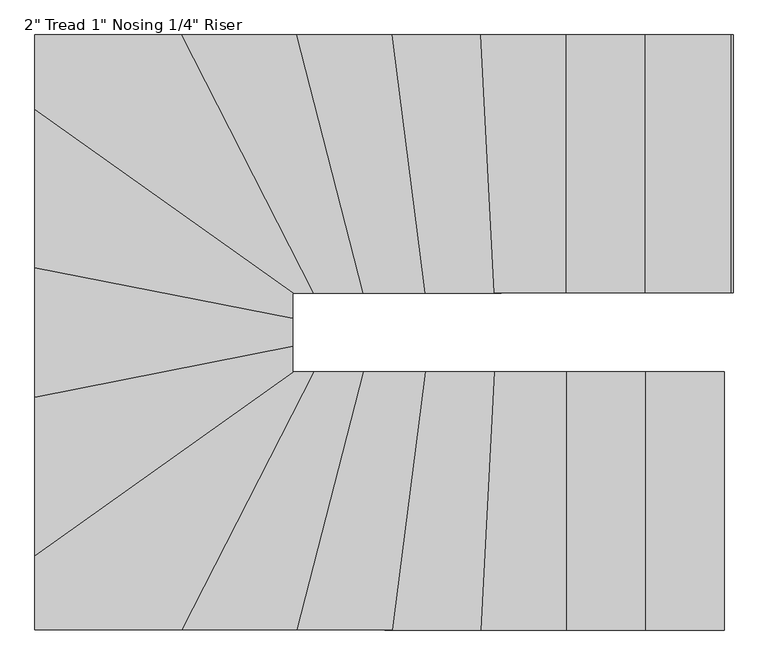
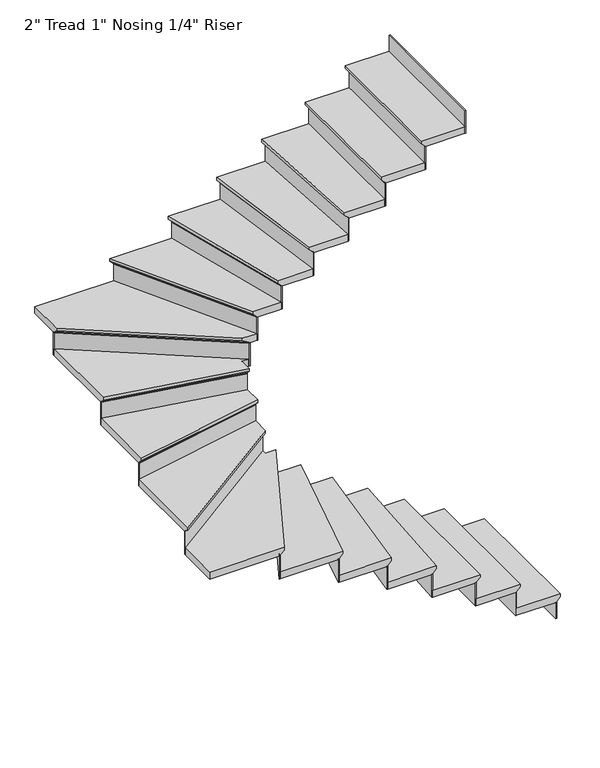
"""IFC4 building model written with IfcOpenShell, lengths in millimetres: stair flight geometry."""

from ifc_helpers import new_model, si_unit, origin, place, context, project, spatial, faceted_brep, source, transform, mapped, element, save


def stair_flight_6f16d7d9(model_context):
    return source(origin(), model_context, "Body", "Brep", [
        faceted_brep([(-1783.4132248, -345.7070853, 150.2833333), (-1783.4132248, -345.7070853, 169.3333333), (-1783.4132248, -1260.1070853, 169.3333333), (-1783.4132248, -1260.1070853, 150.2833333), (-1808.8132248, -345.7070853, 124.8833333), (-1808.8132248, -1260.1070853, 124.8833333), (-2088.2132248, -345.7070853, 169.3333333), (-2088.2132248, -1260.1070853, 169.3333333), (-1808.8132248, -1260.1070853, 118.5333333), (-2088.2132248, -1260.1070853, 118.5333333), (-2088.2132248, -345.7070853, 118.5333333), (-1808.8132248, -345.7070853, 118.5333333)], [[[0, 1, 2, 3]], [[4, 0, 3, 5]], [[2, 1, 6, 7]], [[8, 9, 10, 11]], [[2, 7, 9, 8, 5, 3]], [[8, 11, 4, 5]], [[6, 1, 0, 4, 11, 10]], [[7, 6, 10, 9]]]),
        faceted_brep([(-1808.8132248, -345.7070853, 118.5333333), (-1808.8132248, -345.7070853, 0.0), (-1815.1632248, -345.7070853, 0.0), (-1815.1632248, -345.7070853, 118.5333333), (-1808.8132248, -1260.1070853, 118.5333333), (-1815.1632248, -1260.1070853, 118.5333333), (-1815.1632248, -1260.1070853, 0.0), (-1808.8132248, -1260.1070853, 0.0)], [[[0, 1, 2, 3]], [[4, 5, 6, 7]], [[1, 0, 4, 7]], [[2, 1, 7, 6]], [[3, 2, 6, 5]], [[0, 3, 5, 4]]]),
        faceted_brep([(-2088.2132248, -345.7070853, 287.8666667), (-2088.2132248, -345.7070853, 118.5333333), (-2094.5632248, -345.7070853, 118.5333333), (-2094.5632248, -345.7070853, 287.8666667), (-2088.2132248, -1260.1070853, 287.8666667), (-2094.5632248, -1260.1070853, 287.8666667), (-2094.5632248, -1260.1070853, 118.5333333), (-2088.2132248, -1260.1070853, 118.5333333)], [[[0, 1, 2, 3]], [[4, 5, 6, 7]], [[1, 0, 4, 7]], [[2, 1, 7, 6]], [[3, 2, 6, 5]], [[0, 3, 5, 4]]]),
        faceted_brep([(-2062.8132248, -1260.1070853, 338.6666667), (-2062.8132248, -345.7070853, 338.6666667), (-2367.6132248, -345.7070853, 338.6666667), (-2367.6132248, -1260.1070853, 338.6666667), (-2088.2132248, -1260.1070853, 287.8666667), (-2367.6132248, -1260.1070853, 287.8666667), (-2367.6132248, -345.7070853, 287.8666667), (-2088.2132248, -345.7070853, 287.8666667), (-2088.2132248, -1260.1070853, 294.2166667), (-2062.8132248, -1260.1070853, 319.6166667), (-2088.2132248, -345.7070853, 294.2166667), (-2062.8132248, -345.7070853, 319.6166667)], [[[0, 1, 2, 3]], [[4, 5, 6, 7]], [[0, 3, 5, 4, 8, 9]], [[4, 7, 10, 8]], [[2, 1, 11, 10, 7, 6]], [[3, 2, 6, 5]], [[11, 1, 0, 9]], [[10, 11, 9, 8]]]),
        faceted_brep([(-2367.6132248, -345.7070853, 457.2), (-2367.6132248, -345.7070853, 287.8666667), (-2373.9632248, -345.7070853, 287.8666667), (-2373.9632248, -345.7070853, 457.2), (-2367.6132248, -1260.1070853, 457.2), (-2373.9632248, -1260.1070853, 457.2), (-2373.9632248, -1260.1070853, 287.8666667), (-2367.6132248, -1260.1070853, 287.8666667)], [[[0, 1, 2, 3]], [[4, 5, 6, 7]], [[1, 0, 4, 7]], [[2, 1, 7, 6]], [[3, 2, 6, 5]], [[0, 3, 5, 4]]]),
        faceted_brep([(-2342.2132248, -1260.1070853, 508.0), (-2342.2132248, -345.7070853, 508.0), (-2623.2803863, -345.7070853, 508.0), (-2670.8146567, -1260.1070853, 508.0), (-2367.6132248, -1260.1070853, 457.2), (-2670.8146567, -1260.1070853, 457.2), (-2623.2803863, -345.7070853, 457.2), (-2367.6132248, -345.7070853, 457.2), (-2367.6132248, -1260.1070853, 463.55), (-2342.2132248, -1260.1070853, 488.95), (-2367.6132248, -345.7070853, 463.55), (-2342.2132248, -345.7070853, 488.95)], [[[0, 1, 2, 3]], [[4, 5, 6, 7]], [[0, 3, 5, 4, 8, 9]], [[4, 7, 10, 8]], [[2, 1, 11, 10, 7, 6]], [[3, 2, 6, 5]], [[11, 1, 0, 9]], [[10, 11, 9, 8]]]),
        faceted_brep([(-2623.2803863, -345.7070853, 626.5333333), (-2623.2803863, -345.7070853, 457.2), (-2629.6389604, -345.7070853, 457.2), (-2629.6389604, -345.7070853, 626.5333333), (-2670.8146567, -1260.1070853, 626.5333333), (-2677.1732308, -1260.1070853, 626.5333333), (-2677.1732308, -1260.1070853, 457.2), (-2670.8146567, -1260.1070853, 457.2)], [[[0, 1, 2, 3]], [[4, 5, 6, 7]], [[1, 0, 4, 7]], [[2, 1, 7, 6]], [[3, 2, 6, 5]], [[0, 3, 5, 4]]]),
        faceted_brep([(-2645.38036, -1260.1070853, 677.3333333), (-2597.8460896, -345.7070853, 677.3333333), (-2867.4470861, -345.7070853, 677.3333333), (-2985.8031378, -1260.1070853, 677.3333333), (-2670.8146567, -1260.1070853, 626.5333333), (-2985.8031378, -1260.1070853, 626.5333333), (-2867.4470861, -345.7070853, 626.5333333), (-2623.2803863, -345.7070853, 626.5333333), (-2670.8146567, -1260.1070853, 632.8833333), (-2645.38036, -1260.1070853, 658.2833333), (-2623.2803863, -345.7070853, 632.8833333), (-2597.8460896, -345.7070853, 658.2833333)], [[[0, 1, 2, 3]], [[4, 5, 6, 7]], [[0, 3, 5, 4, 8, 9]], [[4, 7, 10, 8]], [[2, 1, 11, 10, 7, 6]], [[3, 2, 6, 5]], [[11, 1, 0, 9]], [[10, 11, 9, 8]]]),
        faceted_brep([(-2867.4470861, -345.7070853, 795.8666667), (-2867.4470861, -345.7070853, 626.5333333), (-2873.8500579, -345.7070853, 626.5333333), (-2873.8500579, -345.7070853, 795.8666667), (-2985.8031378, -1260.1070853, 795.8666667), (-2992.2061095, -1260.1070853, 795.8666667), (-2992.2061095, -1260.1070853, 626.5333333), (-2985.8031378, -1260.1070853, 626.5333333)], [[[0, 1, 2, 3]], [[4, 5, 6, 7]], [[1, 0, 4, 7]], [[2, 1, 7, 6]], [[3, 2, 6, 5]], [[0, 3, 5, 4]]]),
        faceted_brep([(-2960.1912506, -1260.1070853, 846.6666667), (-2841.835199, -345.7070853, 846.6666667), (-3089.0743086, -345.7070853, 846.6666667), (-3324.204756, -1260.1070853, 846.6666667), (-2985.8031378, -1260.1070853, 795.8666667), (-3324.204756, -1260.1070853, 795.8666667), (-3089.0743086, -345.7070853, 795.8666667), (-2867.4470861, -345.7070853, 795.8666667), (-2985.8031378, -1260.1070853, 802.2166667), (-2960.1912506, -1260.1070853, 827.6166667), (-2867.4470861, -345.7070853, 802.2166667), (-2841.835199, -345.7070853, 827.6166667)], [[[0, 1, 2, 3]], [[4, 5, 6, 7]], [[0, 3, 5, 4, 8, 9]], [[4, 7, 10, 8]], [[2, 1, 11, 10, 7, 6]], [[3, 2, 6, 5]], [[11, 1, 0, 9]], [[10, 11, 9, 8]]]),
        faceted_brep([(-3089.0743086, -345.7070853, 965.2), (-3089.0743086, -345.7070853, 795.8666667), (-3095.6308854, -345.7070853, 795.8666667), (-3095.6308854, -345.7070853, 965.2), (-3324.204756, -1260.1070853, 965.2), (-3330.7613329, -1260.1070853, 965.2), (-3330.7613329, -1260.1070853, 795.8666667), (-3324.204756, -1260.1070853, 795.8666667)], [[[0, 1, 2, 3]], [[4, 5, 6, 7]], [[1, 0, 4, 7]], [[2, 1, 7, 6]], [[3, 2, 6, 5]], [[0, 3, 5, 4]]]),
        faceted_brep([(-3297.9784485, -1260.1070853, 1016.0), (-3062.8480011, -345.7070853, 1016.0), (-3265.4209447, -345.7070853, 1016.0), (-3734.245566, -1260.1070853, 1016.0), (-3324.204756, -1260.1070853, 965.2), (-3734.245566, -1260.1070853, 965.2), (-3265.4209447, -345.7070853, 965.2), (-3089.0743086, -345.7070853, 965.2), (-3324.204756, -1260.1070853, 971.55), (-3297.9784485, -1260.1070853, 996.95), (-3089.0743086, -345.7070853, 971.55), (-3062.8480011, -345.7070853, 996.95)], [[[0, 1, 2, 3]], [[4, 5, 6, 7]], [[0, 3, 5, 4, 8, 9]], [[4, 7, 10, 8]], [[2, 1, 11, 10, 7, 6]], [[3, 2, 6, 5]], [[11, 1, 0, 9]], [[10, 11, 9, 8]]]),
        faceted_brep([(-3265.4209447, -345.7070853, 1134.5333333), (-3265.4209447, -345.7070853, 965.2), (-3272.5569278, -345.7070853, 965.2), (-3272.5569278, -345.7070853, 1134.5333333), (-3734.245566, -1260.1070853, 1134.5333333), (-3741.3815491, -1260.1070853, 1134.5333333), (-3741.3815491, -1260.1070853, 965.2), (-3734.245566, -1260.1070853, 965.2)], [[[0, 1, 2, 3]], [[4, 5, 6, 7]], [[1, 0, 4, 7]], [[2, 1, 7, 6]], [[3, 2, 6, 5]], [[0, 3, 5, 4]]]),
        faceted_brep([(-4225.5449167, -966.4259516, 1185.3333333), (-4225.5449167, -1260.1070853, 1185.3333333), (-3705.7016335, -1260.1070853, 1185.3333333), (-3236.8770121, -345.7070853, 1185.3333333), (-3311.1449167, -345.7070853, 1185.3333333), (-3311.1449167, -316.1520025, 1185.3333333), (-4225.5449167, -1260.1070853, 1134.5333333), (-4225.5449167, -966.4259516, 1134.5333333), (-3311.1449167, -316.1520025, 1134.5333333), (-3311.1449167, -345.7070853, 1134.5333333), (-3265.4209447, -345.7070853, 1134.5333333), (-3734.245566, -1260.1070853, 1134.5333333), (-3734.245566, -1260.1070853, 1140.8833333), (-3705.7016335, -1260.1070853, 1166.2833333), (-3265.4209447, -345.7070853, 1140.8833333), (-3236.8770121, -345.7070853, 1166.2833333)], [[[0, 1, 2, 3, 4, 5]], [[6, 7, 8, 9, 10, 11]], [[1, 0, 7, 6]], [[2, 1, 6, 11, 12, 13]], [[11, 10, 14, 12]], [[4, 3, 15, 14, 10, 9]], [[5, 4, 9, 8]], [[0, 5, 8, 7]], [[15, 3, 2, 13]], [[14, 15, 13, 12]]]),
        faceted_brep([(-3311.1449167, -316.1520025, 1303.8666667), (-3311.1449167, -316.1520025, 1134.5333333), (-3311.1449167, -308.3600277, 1134.5333333), (-3311.1449167, -308.3600277, 1303.8666667), (-4225.5449167, -966.4259516, 1303.8666667), (-4225.5449167, -958.6339768, 1303.8666667), (-4225.5449167, -958.6339768, 1134.5333333), (-4225.5449167, -966.4259516, 1134.5333333)], [[[0, 1, 2, 3]], [[4, 5, 6, 7]], [[1, 0, 4, 7]], [[2, 1, 7, 6]], [[3, 2, 6, 5]], [[0, 3, 5, 4]]]),
        faceted_brep([(-4225.5449167, -997.5938508, 1354.6666667), (-3311.1449167, -347.3199017, 1354.6666667), (-3311.1449167, -229.6979154, 1354.6666667), (-4225.5449167, -409.9387717, 1354.6666667), (-4225.5449167, -966.4259516, 1303.8666667), (-4225.5449167, -409.9387717, 1303.8666667), (-3311.1449167, -229.6979154, 1303.8666667), (-3311.1449167, -316.1520025, 1303.8666667), (-4225.5449167, -966.4259516, 1310.2166667), (-4225.5449167, -997.5938508, 1335.6166667), (-3311.1449167, -316.1520025, 1310.2166667), (-3311.1449167, -347.3199017, 1335.6166667)], [[[0, 1, 2, 3]], [[4, 5, 6, 7]], [[0, 3, 5, 4, 8, 9]], [[4, 7, 10, 8]], [[2, 1, 11, 10, 7, 6]], [[3, 2, 6, 5]], [[11, 1, 0, 9]], [[10, 11, 9, 8]]]),
        faceted_brep([(-3311.1449167, -229.6979154, 1473.2), (-3311.1449167, -229.6979154, 1303.8666667), (-3311.1449167, -223.22573, 1303.8666667), (-3311.1449167, -223.22573, 1473.2), (-4225.5449167, -409.9387717, 1473.2), (-4225.5449167, -403.4665863, 1473.2), (-4225.5449167, -403.4665863, 1303.8666667), (-4225.5449167, -409.9387717, 1303.8666667)], [[[0, 1, 2, 3]], [[4, 5, 6, 7]], [[1, 0, 4, 7]], [[2, 1, 7, 6]], [[3, 2, 6, 5]], [[0, 3, 5, 4]]]),
        faceted_brep([(-4225.5449167, -435.8275135, 1524.0), (-3311.1449167, -255.5866572, 1524.0), (-3311.1449167, -130.5387717, 1524.0), (-4225.5449167, 49.7020846, 1524.0), (-4225.5449167, -409.9387717, 1473.2), (-4225.5449167, 49.7020846, 1473.2), (-3311.1449167, -130.5387717, 1473.2), (-3311.1449167, -229.6979154, 1473.2), (-4225.5449167, -409.9387717, 1479.55), (-4225.5449167, -435.8275135, 1504.95), (-3311.1449167, -229.6979154, 1479.55), (-3311.1449167, -255.5866572, 1504.95)], [[[0, 1, 2, 3]], [[4, 5, 6, 7]], [[0, 3, 5, 4, 8, 9]], [[4, 7, 10, 8]], [[2, 1, 11, 10, 7, 6]], [[3, 2, 6, 5]], [[11, 1, 0, 9]], [[10, 11, 9, 8]]]),
        faceted_brep([(-3311.1449167, -130.5387717, 1642.5333333), (-3311.1449167, -130.5387717, 1473.2), (-3311.1449167, -124.0665863, 1473.2), (-3311.1449167, -124.0665863, 1642.5333333), (-4225.5449167, 49.7020846, 1642.5333333), (-4225.5449167, 56.17427, 1642.5333333), (-4225.5449167, 56.17427, 1473.2), (-4225.5449167, 49.7020846, 1473.2)], [[[0, 1, 2, 3]], [[4, 5, 6, 7]], [[1, 0, 4, 7]], [[2, 1, 7, 6]], [[3, 2, 6, 5]], [[0, 3, 5, 4]]]),
        faceted_brep([(-4225.5449167, 23.8133428, 1693.3333333), (-3311.1449167, -156.4275135, 1693.3333333), (-3311.1449167, -66.3070853, 1693.3333333), (-3265.0494422, -66.3070853, 1693.3333333), (-4225.5449167, 616.7475793, 1693.3333333), (-4225.5449167, 49.7020846, 1642.5333333), (-4225.5449167, 616.7475793, 1642.5333333), (-3265.0494422, -66.3070853, 1642.5333333), (-3311.1449167, -66.3070853, 1642.5333333), (-3311.1449167, -130.5387717, 1642.5333333), (-4225.5449167, 49.7020846, 1648.8833333), (-4225.5449167, 23.8133428, 1674.2833333), (-3311.1449167, -130.5387717, 1648.8833333), (-3311.1449167, -156.4275135, 1674.2833333)], [[[0, 1, 2, 3, 4]], [[5, 6, 7, 8, 9]], [[0, 4, 6, 5, 10, 11]], [[5, 9, 12, 10]], [[2, 1, 13, 12, 9, 8]], [[3, 2, 8, 7]], [[4, 3, 7, 6]], [[13, 1, 0, 11]], [[12, 13, 11, 10]]]),
        faceted_brep([(-3265.0494422, -66.3070853, 1811.8666667), (-3265.0494422, -66.3070853, 1642.5333333), (-3254.0925497, -66.3070853, 1642.5333333), (-3254.0925497, -66.3070853, 1811.8666667), (-4225.5449167, 616.7475793, 1811.8666667), (-4225.5449167, 624.5395541, 1811.8666667), (-4225.5449167, 624.5395541, 1642.5333333), (-4225.5449167, 616.7475793, 1642.5333333)], [[[0, 1, 2, 3]], [[4, 5, 6, 7]], [[1, 0, 4, 7]], [[2, 1, 7, 6]], [[3, 2, 6, 5]], [[0, 3, 5, 4]]]),
        faceted_brep([(-3677.1577009, 848.0929147, 1862.6666667), (-4225.5449167, 848.0929147, 1862.6666667), (-4225.5449167, 585.5796802, 1862.6666667), (-3308.8770121, -66.3070853, 1862.6666667), (-3208.3330796, -66.3070853, 1862.6666667), (-4225.5449167, 848.0929147, 1811.8666667), (-3677.1577009, 848.0929147, 1811.8666667), (-3208.3330796, -66.3070853, 1811.8666667), (-3265.0494422, -66.3070853, 1811.8666667), (-4225.5449167, 616.7475793, 1811.8666667), (-4225.5449167, 616.7475793, 1818.2166667), (-4225.5449167, 585.5796802, 1843.6166667), (-3265.0494422, -66.3070853, 1818.2166667), (-3308.8770121, -66.3070853, 1843.6166667)], [[[0, 1, 2, 3, 4]], [[5, 6, 7, 8, 9]], [[1, 0, 6, 5]], [[2, 1, 5, 9, 10, 11]], [[9, 8, 12, 10]], [[4, 3, 13, 12, 8, 7]], [[0, 4, 7, 6]], [[13, 3, 2, 11]], [[12, 13, 11, 10]]]),
        faceted_brep([(-3208.3330796, -66.3070853, 1981.2), (-3208.3330796, -66.3070853, 1811.8666667), (-3201.1970965, -66.3070853, 1811.8666667), (-3201.1970965, -66.3070853, 1981.2), (-3677.1577009, 848.0929147, 1981.2), (-3670.0217178, 848.0929147, 1981.2), (-3670.0217178, 848.0929147, 1811.8666667), (-3677.1577009, 848.0929147, 1811.8666667)], [[[0, 1, 2, 3]], [[4, 5, 6, 7]], [[1, 0, 4, 7]], [[2, 1, 7, 6]], [[3, 2, 6, 5]], [[0, 3, 5, 4]]]),
        faceted_brep([(-3705.7016335, 848.0929147, 2032.0), (-3236.8770121, -66.3070853, 2032.0), (-3036.6216937, -66.3070853, 2032.0), (-3271.7521411, 848.0929147, 2032.0), (-3677.1577009, 848.0929147, 1981.2), (-3271.7521411, 848.0929147, 1981.2), (-3036.6216937, -66.3070853, 1981.2), (-3208.3330796, -66.3070853, 1981.2), (-3677.1577009, 848.0929147, 1987.55), (-3705.7016335, 848.0929147, 2012.95), (-3208.3330796, -66.3070853, 1987.55), (-3236.8770121, -66.3070853, 2012.95)], [[[0, 1, 2, 3]], [[4, 5, 6, 7]], [[0, 3, 5, 4, 8, 9]], [[4, 7, 10, 8]], [[2, 1, 11, 10, 7, 6]], [[3, 2, 6, 5]], [[11, 1, 0, 9]], [[10, 11, 9, 8]]]),
        faceted_brep([(-3036.6216937, -66.3070853, 2150.5333333), (-3036.6216937, -66.3070853, 1981.2), (-3030.0651168, -66.3070853, 1981.2), (-3030.0651168, -66.3070853, 2150.5333333), (-3271.7521411, 848.0929147, 2150.5333333), (-3265.1955642, 848.0929147, 2150.5333333), (-3265.1955642, 848.0929147, 1981.2), (-3271.7521411, 848.0929147, 1981.2)], [[[0, 1, 2, 3]], [[4, 5, 6, 7]], [[1, 0, 4, 7]], [[2, 1, 7, 6]], [[3, 2, 6, 5]], [[0, 3, 5, 4]]]),
        faceted_brep([(-3297.9784485, 848.0929147, 2201.3333333), (-3062.8480011, -66.3070853, 2201.3333333), (-2816.2233119, -66.3070853, 2201.3333333), (-2934.5793635, 848.0929147, 2201.3333333), (-3271.7521411, 848.0929147, 2150.5333333), (-2934.5793635, 848.0929147, 2150.5333333), (-2816.2233119, -66.3070853, 2150.5333333), (-3036.6216937, -66.3070853, 2150.5333333), (-3271.7521411, 848.0929147, 2156.8833333), (-3297.9784485, 848.0929147, 2182.2833333), (-3036.6216937, -66.3070853, 2156.8833333), (-3062.8480011, -66.3070853, 2182.2833333)], [[[0, 1, 2, 3]], [[4, 5, 6, 7]], [[0, 3, 5, 4, 8, 9]], [[4, 7, 10, 8]], [[2, 1, 11, 10, 7, 6]], [[3, 2, 6, 5]], [[11, 1, 0, 9]], [[10, 11, 9, 8]]]),
        faceted_brep([(-2816.2233119, -66.3070853, 2319.8666667), (-2816.2233119, -66.3070853, 2150.5333333), (-2809.8203401, -66.3070853, 2150.5333333), (-2809.8203401, -66.3070853, 2319.8666667), (-2934.5793635, 848.0929147, 2319.8666667), (-2928.1763918, 848.0929147, 2319.8666667), (-2928.1763918, 848.0929147, 2150.5333333), (-2934.5793635, 848.0929147, 2150.5333333)], [[[0, 1, 2, 3]], [[4, 5, 6, 7]], [[1, 0, 4, 7]], [[2, 1, 7, 6]], [[3, 2, 6, 5]], [[0, 3, 5, 4]]]),
        faceted_brep([(-2960.1912506, 848.0929147, 2370.6666667), (-2841.835199, -66.3070853, 2370.6666667), (-2572.411793, -66.3070853, 2370.6666667), (-2619.9460634, 848.0929147, 2370.6666667), (-2934.5793635, 848.0929147, 2319.8666667), (-2619.9460634, 848.0929147, 2319.8666667), (-2572.411793, -66.3070853, 2319.8666667), (-2816.2233119, -66.3070853, 2319.8666667), (-2934.5793635, 848.0929147, 2326.2166667), (-2960.1912506, 848.0929147, 2351.6166667), (-2816.2233119, -66.3070853, 2326.2166667), (-2841.835199, -66.3070853, 2351.6166667)], [[[0, 1, 2, 3]], [[4, 5, 6, 7]], [[0, 3, 5, 4, 8, 9]], [[4, 7, 10, 8]], [[2, 1, 11, 10, 7, 6]], [[3, 2, 6, 5]], [[11, 1, 0, 9]], [[10, 11, 9, 8]]]),
        faceted_brep([(-2572.411793, -66.3070853, 2489.2), (-2572.411793, -66.3070853, 2319.8666667), (-2566.0532188, -66.3070853, 2319.8666667), (-2566.0532188, -66.3070853, 2489.2), (-2619.9460634, 848.0929147, 2489.2), (-2613.5874892, 848.0929147, 2489.2), (-2613.5874892, 848.0929147, 2319.8666667), (-2619.9460634, 848.0929147, 2319.8666667)], [[[0, 1, 2, 3]], [[4, 5, 6, 7]], [[1, 0, 4, 7]], [[2, 1, 7, 6]], [[3, 2, 6, 5]], [[0, 3, 5, 4]]]),
        faceted_brep([(-2645.38036, 848.0929147, 2540.0), (-2597.8460896, -66.3070853, 2540.0), (-2316.8132248, -66.3070853, 2540.0), (-2316.8132248, 848.0929147, 2540.0), (-2619.9460634, 848.0929147, 2489.2), (-2316.8132248, 848.0929147, 2489.2), (-2316.8132248, -66.3070853, 2489.2), (-2572.411793, -66.3070853, 2489.2), (-2619.9460634, 848.0929147, 2495.55), (-2645.38036, 848.0929147, 2520.95), (-2572.411793, -66.3070853, 2495.55), (-2597.8460896, -66.3070853, 2520.95)], [[[0, 1, 2, 3]], [[4, 5, 6, 7]], [[0, 3, 5, 4, 8, 9]], [[4, 7, 10, 8]], [[2, 1, 11, 10, 7, 6]], [[3, 2, 6, 5]], [[11, 1, 0, 9]], [[10, 11, 9, 8]]]),
        faceted_brep([(-2316.8132248, -66.3070853, 2658.5333333), (-2316.8132248, -66.3070853, 2489.2), (-2310.4632248, -66.3070853, 2489.2), (-2310.4632248, -66.3070853, 2658.5333333), (-2316.8132248, 848.0929147, 2658.5333333), (-2310.4632248, 848.0929147, 2658.5333333), (-2310.4632248, 848.0929147, 2489.2), (-2316.8132248, 848.0929147, 2489.2)], [[[0, 1, 2, 3]], [[4, 5, 6, 7]], [[1, 0, 4, 7]], [[2, 1, 7, 6]], [[3, 2, 6, 5]], [[0, 3, 5, 4]]]),
        faceted_brep([(-2342.2132248, 848.0929147, 2709.3333333), (-2342.2132248, -66.3070853, 2709.3333333), (-2037.4132248, -66.3070853, 2709.3333333), (-2037.4132248, 848.0929147, 2709.3333333), (-2316.8132248, 848.0929147, 2658.5333333), (-2037.4132248, 848.0929147, 2658.5333333), (-2037.4132248, -66.3070853, 2658.5333333), (-2316.8132248, -66.3070853, 2658.5333333), (-2316.8132248, 848.0929147, 2664.8833333), (-2342.2132248, 848.0929147, 2690.2833333), (-2316.8132248, -66.3070853, 2664.8833333), (-2342.2132248, -66.3070853, 2690.2833333)], [[[0, 1, 2, 3]], [[4, 5, 6, 7]], [[0, 3, 5, 4, 8, 9]], [[4, 7, 10, 8]], [[2, 1, 11, 10, 7, 6]], [[3, 2, 6, 5]], [[11, 1, 0, 9]], [[10, 11, 9, 8]]]),
        faceted_brep([(-2037.4132248, -66.3070853, 2827.8666667), (-2037.4132248, -66.3070853, 2658.5333333), (-2031.0632248, -66.3070853, 2658.5333333), (-2031.0632248, -66.3070853, 2827.8666667), (-2037.4132248, 848.0929147, 2827.8666667), (-2031.0632248, 848.0929147, 2827.8666667), (-2031.0632248, 848.0929147, 2658.5333333), (-2037.4132248, 848.0929147, 2658.5333333)], [[[0, 1, 2, 3]], [[4, 5, 6, 7]], [[1, 0, 4, 7]], [[2, 1, 7, 6]], [[3, 2, 6, 5]], [[0, 3, 5, 4]]]),
        faceted_brep([(-1758.0132248, -66.3070853, 2997.2), (-1758.0132248, -66.3070853, 2827.8666667), (-1751.6632248, -66.3070853, 2827.8666667), (-1751.6632248, -66.3070853, 2997.2), (-1758.0132248, 848.0929147, 2997.2), (-1751.6632248, 848.0929147, 2997.2), (-1751.6632248, 848.0929147, 2827.8666667), (-1758.0132248, 848.0929147, 2827.8666667)], [[[0, 1, 2, 3]], [[4, 5, 6, 7]], [[1, 0, 4, 7]], [[2, 1, 7, 6]], [[3, 2, 6, 5]], [[0, 3, 5, 4]]]),
        faceted_brep([(-2062.8132248, 848.0929147, 2878.6666667), (-2062.8132248, -66.3070853, 2878.6666667), (-1758.0132248, -66.3070853, 2878.6666667), (-1758.0132248, 848.0929147, 2878.6666667), (-2037.4132248, 848.0929147, 2827.8666667), (-1758.0132248, 848.0929147, 2827.8666667), (-1758.0132248, -66.3070853, 2827.8666667), (-2037.4132248, -66.3070853, 2827.8666667), (-2037.4132248, 848.0929147, 2834.2166667), (-2062.8132248, 848.0929147, 2859.6166667), (-2037.4132248, -66.3070853, 2834.2166667), (-2062.8132248, -66.3070853, 2859.6166667)], [[[0, 1, 2, 3]], [[4, 5, 6, 7]], [[0, 3, 5, 4, 8, 9]], [[4, 7, 10, 8]], [[2, 1, 11, 10, 7, 6]], [[3, 2, 6, 5]], [[11, 1, 0, 9]], [[10, 11, 9, 8]]]),
    ])


if __name__ == "__main__":
    model = new_model("IFC4")
    model_context = context("Model", 3, world=origin())
    ifc_project = project(units=[si_unit("LENGTHUNIT", "METRE", prefix="MILLI")], contexts=[model_context])
    site = spatial("IfcSite", under=ifc_project)
    building = spatial("IfcBuilding", under=site)
    placement = place(None, origin())
    stair_flight_shape = stair_flight_6f16d7d9(model_context)
    element("IfcStairFlight", 1, ObjectType="2\" Tread 1\" Nosing 1/4\" Riser", at=placement, inside=building, context=model_context, shape_type="MappedRepresentation", body=[
        mapped(stair_flight_shape, transform((0.0, 0.0, 0.0), x_axis=(1.0, 0.0, 0.0), y_axis=(0.0, 1.0, 0.0), z_axis=(0.0, 0.0, 1.0))),
    ])
    save(model, "model.ifc")
